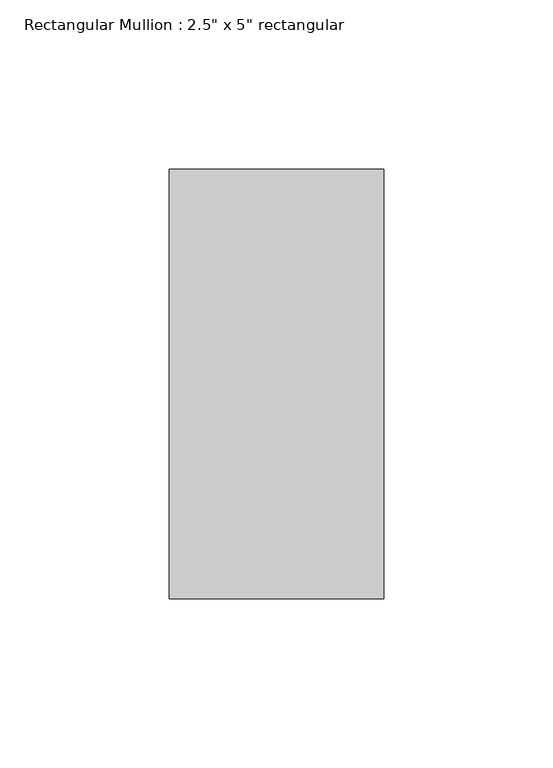
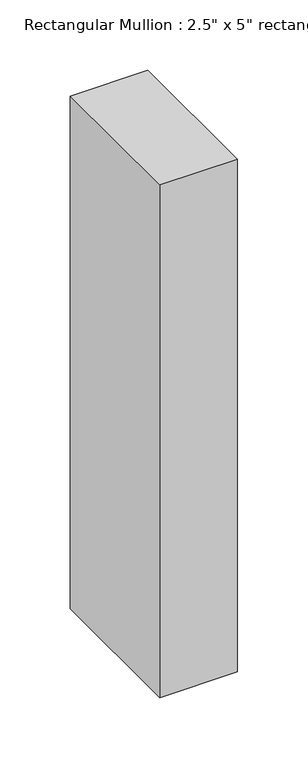
"""IFC4 building model written with IfcOpenShell, lengths in millimetres: member geometry."""

from ifc_helpers import new_model, si_unit, frame, origin, place, context, project, spatial, polyline, outline, extrude, source, transform, mapped, element, save


def member_718fe5d9(model_context):
    return source(origin(), model_context, "Body", "SweptSolid", [
        extrude(outline(polyline([(31.75, 63.5), (31.75, -63.5), (-31.75, -63.5), (-31.75, 63.5), (31.75, 63.5)])), frame((0.0, 0.0, -444.5), z_axis=(0.0, 0.0, 1.0), x_axis=(1.0, 0.0, 0.0)), (0.0, 0.0, 1.0), 444.5),
    ])


if __name__ == "__main__":
    model = new_model("IFC4")
    model_context = context("Model", 3, world=origin())
    ifc_project = project(units=[si_unit("LENGTHUNIT", "METRE", prefix="MILLI")], contexts=[model_context])
    site = spatial("IfcSite", under=ifc_project)
    building = spatial("IfcBuilding", under=site)
    placement = place(None, origin())
    member_shape = member_718fe5d9(model_context)
    element("IfcMember", 1, ObjectType="Rectangular Mullion : 2.5\" x 5\" rectangular", at=placement, inside=building, context=model_context, shape_type="MappedRepresentation", body=[
        mapped(member_shape, transform((0.0, 0.0, 0.0), x_axis=(1.0, 0.0, 0.0), y_axis=(0.0, 1.0, 0.0), z_axis=(0.0, 0.0, 1.0))),
    ])
    save(model, "model.ifc")

# Revit data of these elements
# Type "Rectangular Mullion : 2.5\" x 5\" rectangular"
#   built-in parameter 1007304 = 0.416667 (stored number, unit not read)
#   built-in parameter 1007301 = 0.104167 (stored number, unit not read)
#   built-in parameter 1007300 = 0.104167 (stored number, unit not read)
# Element 1 (IfcMember, "Rectangular Mullion : 2.5\" x 5\" rectangular")
#   Materials on its faces: "door colour"
# Materials
#   "door colour": class "Generic", colour RGB 120 120 120, transparency 0, Cost = 0
